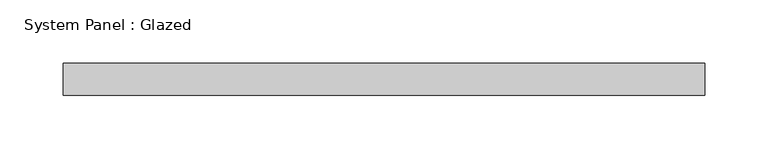
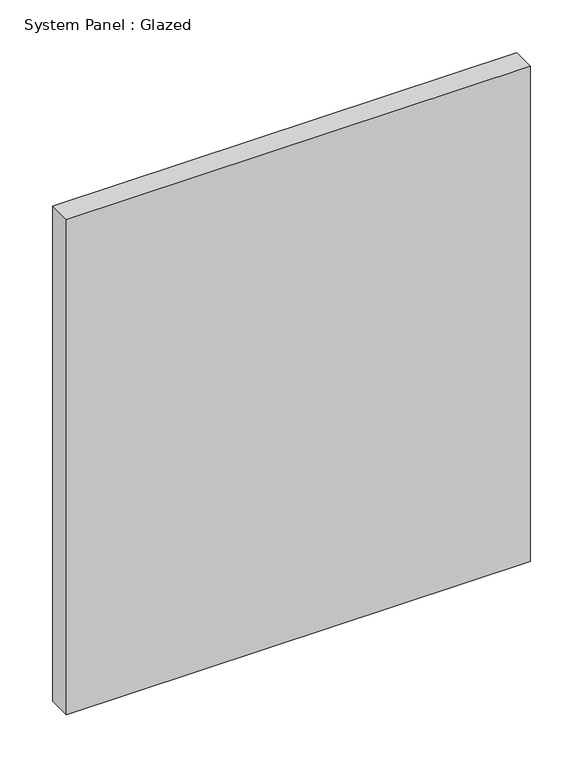
"""IFC4 building model written with IfcOpenShell, lengths in millimetres: plate geometry, System Panel : Glazed."""

from ifc_helpers import new_model, si_unit, origin, origin_with_axes, place, context, project, spatial, polyline, outline, extrude, source, transform, mapped, element, save


def system_panel_glazed_f2280d1b(model_context):
    return source(origin(), model_context, "Body", "SweptSolid", [
        extrude(outline(polyline([(254.0, 19.05), (-254.0, 19.05), (-254.0, 44.45), (254.0, 44.45), (254.0, 19.05)])), origin_with_axes(), (0.0, 0.0, 1.0), 573.4647936),
    ])


if __name__ == "__main__":
    model = new_model("IFC4")
    model_context = context("Model", 3, world=origin())
    ifc_project = project(units=[si_unit("LENGTHUNIT", "METRE", prefix="MILLI")], contexts=[model_context])
    site = spatial("IfcSite", under=ifc_project)
    building = spatial("IfcBuilding", under=site)
    placement = place(None, origin())
    system_panel_glazed_shape = system_panel_glazed_f2280d1b(model_context)
    element("IfcPlate", 1, ObjectType="System Panel : Glazed", at=placement, inside=building, context=model_context, shape_type="MappedRepresentation", body=[
        mapped(system_panel_glazed_shape, transform((0.0, 0.0, 0.0), x_axis=(1.0, 0.0, 0.0), y_axis=(0.0, 1.0, 0.0), z_axis=(0.0, 0.0, 1.0))),
    ])
    save(model, "model.ifc")

# Revit data of these elements
# Type "System Panel : Glazed"
#   Construction Type Id = "GSP4R"
#   Analytic Construction = "1/8 in Pilkington single glazing"
#   Visual Light Transmittance = 0.9
#   Solar Heat Gain Coefficient = 0.86
#   Heat Transfer Coefficient (U) = 1.18115 BTU/(h·ft²·°F)
#   Define Thermal Properties by = 1
# Element 1 (IfcPlate, "System Panel : Glazed")
#   Materials on its faces: "Glass"
# Materials
#   "Glass": class "Glass", colour RGB 0 128 192, transparency 0.75, Description = "Soda Lime Glass", Cost = 0
